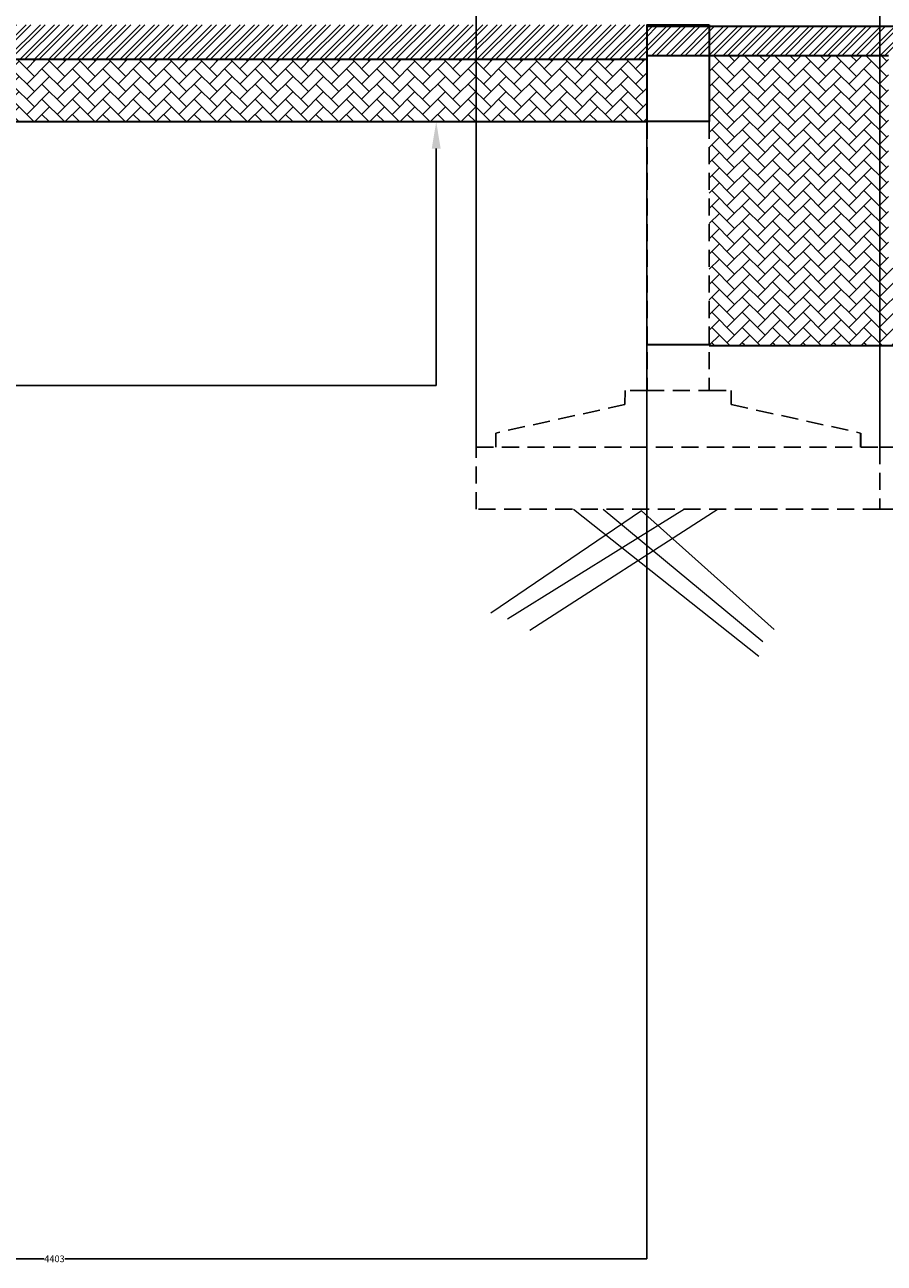
# Model space of a CAD drawing. Units: millimetres. Extents: x 1944 to 29915, y -10550 to 5909.
# Tile 19 of 24: x 22846 to 26040, y -10550 to -5946. Entities that reach past the tile are written whole.
import ezdxf
from ezdxf import colors
from ezdxf.entities.mleader import LeaderData, LeaderLine
from ezdxf.math import Vec2, Vec3

# ---------------------------------------------------------------- set-up
doc = ezdxf.new("R2010")
doc.units = ezdxf.units.MM
doc.header["$MEASUREMENT"] = 0
doc.linetypes.add('HIDDEN', pattern=[9.525, 6.35, -3.175])
for name, color, linetype, lineweight in [('A-ANNO-DIMS', 2, 'Continuous', 18), ('A-ANNO-TEXT', 7, 'Continuous', 25), ('A-FLOR-PATT', 252, 'Continuous', 13), ('A-SECT', 7, 'Continuous', 35), ('C-TOPO', 94, 'Continuous', 18), ('S-FNDN-HIDN', 1, 'HIDDEN', 25)]:
    doc.layers.add(name, color=color, linetype=linetype, lineweight=lineweight)
doc.styles.get("Standard").update_dxf_attribs({"font": 'arial.ttf'})
doc.dimstyles.get("Standard").update_dxf_attribs({"dimtxt": 25, "dimasz": 0.18, "dimexe": 0.18, "dimexo": 0.0625, "dimgap": 0.09, "dimtad": 0, "dimtih": 1, "dimtoh": 1, "dimdec": 0, "dimzin": 0, "dimdsep": 46, "dimtxsty": 'Standard', "dimcen": 0.09, "dimadec": 0, "dimazin": 0, "dimtfac": 1, "dimtdec": 0, "dimtofl": 0, "dimtmove": 0, "dimatfit": 3, "dimfxl": 1, "dimtolj": 1, "dimtzin": 0, "dimarcsym": 0})

# ---------------------------------------------------------------- blocks, each defined once
blk = doc.blocks.new('EARTH-COMPACT-SYMB')
for q in [(0, 60.9), (1053, 0)]:
    blk.add_line((559.8, 441.1), q)
blk = doc.blocks.new('*D89')
at = {"layer": 'A-ANNO-DIMS', "color": 0, "lineweight": -2, "transparency": 16777216}
for p, q in [((20755.4, -6305.8), (20755.4, -10533.3)), ((25158, -6305.8), (25158, -10533.3)), ((20755.6, -10533.1), (22918.8, -10533.1)), ((25157.8, -10533.1), (22994.7, -10533.1))]:
    blk.add_line(p, q, dxfattribs=at)
at = {"layer": 'A-ANNO-DIMS', "color": 0, "transparency": 16777216}
for points in [[(20755.6, -10533.1), (20755.6, -10533.1), (20755.4, -10533.1)], [(25157.8, -10533.1), (25157.8, -10533.1), (25158, -10533.1)]]:
    blk.add_solid(points, dxfattribs=at)
at = {"layer": 'Defpoints', "color": 0, "transparency": 16777216}
for p in [(20755.4, -6305.8), (25158, -6305.8), (25158, -10533.1)]:
    blk.add_point(p, dxfattribs=at)
at = {"layer": 'A-ANNO-DIMS', "color": 0, "transparency": 16777216, "insert": (22956.7, -10533.1), "char_height": 25, "attachment_point": 5}
blk.add_mtext('\\A1;4403', dxfattribs=at)
blk = doc.blocks.new('*D91')
at = {"layer": 'A-ANNO-DIMS', "color": 0, "lineweight": -2, "transparency": 16777216}
for p, q in [((24524.3, -7516.2), (24524.3, -395.6)), ((24524.5, -395.8), (25238.1, -395.8)), ((26024.1, -395.8), (25310.5, -395.8)), ((26024.3, -7516.2), (26024.3, -395.6))]:
    blk.add_line(p, q, dxfattribs=at)
at = {"layer": 'A-ANNO-DIMS', "color": 0, "transparency": 16777216}
for points in [[(24524.5, -395.7), (24524.5, -395.8), (24524.3, -395.8)], [(26024.1, -395.7), (26024.1, -395.8), (26024.3, -395.8)]]:
    blk.add_solid(points, dxfattribs=at)
at = {"layer": 'Defpoints', "color": 0, "transparency": 16777216}
for p in [(26024.3, -395.8), (24524.3, -7516.2), (26024.3, -7516.2)]:
    blk.add_point(p, dxfattribs=at)
at = {"layer": 'A-ANNO-DIMS', "color": 0, "transparency": 16777216, "insert": (25274.3, -395.8), "char_height": 25, "attachment_point": 5}
blk.add_mtext('\\A1;1500', dxfattribs=at)
blk = doc.blocks.new('*D92')
at = {"layer": 'A-ANNO-DIMS', "color": 0, "lineweight": -2, "transparency": 16777216}
for p, q in [((26024.4, -7516.2), (29886.4, -7516.2)), ((29886.2, -7516.4), (29886.2, -7618.4)), ((29886.2, -7746), (29886.2, -7644.1)), ((26024.4, -7746.2), (29886.4, -7746.2))]:
    blk.add_line(p, q, dxfattribs=at)
at = {"layer": 'A-ANNO-DIMS', "color": 0, "transparency": 16777216}
for points in [[(29886.2, -7516.4), (29886.3, -7516.4), (29886.2, -7516.2)], [(29886.2, -7746), (29886.3, -7746), (29886.2, -7746.2)]]:
    blk.add_solid(points, dxfattribs=at)
at = {"layer": 'Defpoints', "color": 0, "transparency": 16777216}
for p in [(26024.3, -7516.2), (26024.3, -7746.2), (29886.2, -7746.2)]:
    blk.add_point(p, dxfattribs=at)
at = {"layer": 'A-ANNO-DIMS', "color": 0, "transparency": 16777216, "insert": (29886.2, -7631.2), "char_height": 25, "attachment_point": 5}
blk.add_mtext('\\A1;230', dxfattribs=at)

msp = doc.modelspace()

# ---------------------------------------------------------------- hatches: boundary and pattern name
at = {"layer": 'A-FLOR-PATT'}
h = msp.add_hatch(dxfattribs=at)
h.set_pattern_fill('ANSI32', color=256, scale=100)
h.paths.add_polyline_path([(25159.297, -5945.752), (20985.45, -5945.752), (20985.45, -6073.852), (25159.297, -6073.852)])
h = msp.add_hatch(dxfattribs=at)
h.set_pattern_fill('ANSI32', color=256, scale=100)
h.paths.add_polyline_path([(25158.02, -5950.967), (26236.262, -5950.967), (26332.914, -6053.056), (26056.262, -6061.05), (25158.02, -6061.05)])
h = msp.add_hatch(dxfattribs=at)
h.set_pattern_fill('AR-HBONE', color=256, scale=10)
h.paths.add_polyline_path([(25159.297, -6073.852), (20985.45, -6073.852), (20985.45, -6305.752), (25159.297, -6305.752)])
h = msp.add_hatch(dxfattribs=at)
h.set_pattern_fill('AR-HBONE', color=256, scale=10)
h.paths.add_polyline_path([(25389.297, -6305.752), (25389.297, -6061.05), (26056.262, -6061.05), (26056.262, -6850.967), (26236.262, -6850.967), (27005.891, -6850.967), (27005.891, -6990.545), (26995.108, -6990.545), (26995.108, -7135.877), (25389.297, -7135.877)])

# ---------------------------------------------------------------- linework, layer by layer
at = {"layer": 'A-SECT'}
for p, q in [((25158.02, -5950.967), (26236.262, -5950.967)), ((20985.45, -6073.852), (25159.297, -6073.852)), ((26056.262, -6061.05), (25158.02, -6061.05)), ((20985.45, -6305.752), (25159.297, -6305.752)), ((25389.297, -7135.877), (25158.02, -7135.877)), ((27005.891, -7139.615), (25389.297, -7139.615)), ((25951.921, -7463.338), (25951.921, -7516.218))]:
    msp.add_line(p, q, dxfattribs=at)
msp.add_lwpolyline([(25389.297, -5945.752), (25389.297, -6305.752), (25159.297, -6305.752), (25159.297, -5945.752), (25389.297, -5945.752)], dxfattribs=at)
at = {"layer": 'C-TOPO'}
for p, q in [((25298.094, -7746.218), (24639.796, -8155.847)), ((25423.049, -7746.218), (24723.607, -8196.963)), ((24885.134, -7746.218), (25573.909, -8292.9)), ((24996.374, -7746.218), (25589.148, -8238.079))]:
    msp.add_line(p, q, dxfattribs=at)
at = {"layer": 'S-FNDN-HIDN', "ltscale": 10}
for p, q in [((25158.02, -6305.752), (25158.02, -7305.752)), ((25159.297, -6305.752), (25159.297, -7305.752)), ((25389.297, -6305.752), (25389.297, -7305.752)), ((25077.268, -7304.748), (25076.626, -7357.264)), ((25159.297, -7305.752), (25077.268, -7304.748)), ((25158.02, -7305.752), (25240.049, -7304.748)), ((25159.297, -7305.752), (25389.297, -7305.752)), ((25389.297, -7305.752), (25471.326, -7304.748)), ((25471.326, -7304.748), (25471.968, -7357.264)), ((25076.626, -7357.264), (24596.673, -7463.338)), ((25471.968, -7357.264), (25951.921, -7463.338)), ((24596.673, -7463.338), (24596.673, -7516.218))]:
    msp.add_line(p, q, dxfattribs=at)
msp.add_lwpolyline([(24524.297, -7516.218), (26024.297, -7516.218), (26024.297, -7746.218), (24524.297, -7746.218)], close=True, dxfattribs=at)

# ---------------------------------------------------------------- block references
at = {"layer": 'C-TOPO'}
msp.add_blockref('EARTH-COMPACT-SYMB', (24578.843, -8193.917), dxfattribs=at)

# ---------------------------------------------------------------- dimensions: what is measured, and where the dimension line sits
at = {"layer": 'A-ANNO-DIMS'}
for base, p1, p2, picture, middle in [((26024.297, -395.752), (24524.297, -7516.218), (26024.297, -7516.218), '*D91', (25274.297, -395.752)), ((25158.02, -10533.115), (20755.45, -6305.752), (25158.02, -6305.752), '*D89', (22956.735, -10533.115))]:
    dim = msp.add_linear_dim(base=base, p1=p1, p2=p2, dimstyle='Standard', override={"dimdec": 0, "dimlfac": 1, "dimrnd": 0, "dimzin": 0, "dimdsep": 46, "dimlunit": 2}, dxfattribs=at)
    dim.commit()
    dim.dimension.update_dxf_attribs({"geometry": picture, "text_midpoint": middle})
dim = msp.add_linear_dim(base=(29886.248, -7746.218), p1=(26024.297, -7516.218), p2=(26024.297, -7746.218), angle=90, dimstyle='Standard', override={"dimdec": 0, "dimlfac": 1, "dimrnd": 0, "dimzin": 0, "dimdsep": 46, "dimlunit": 2}, dxfattribs=at)
dim.commit()
dim.dimension.update_dxf_attribs({"geometry": '*D92', "text_midpoint": (29886.248, -7631.218)})

# ---------------------------------------------------------------- leaders
at = {"layer": 'A-ANNO-TEXT'}
ml = msp.add_multileader_mtext('Standard', dxfattribs=at)
ml.set_content('COMPACTED EARETH ', color=256)
ml.set_leader_properties()
ml.build(insert=Vec2(0, 0))
ml.multileader.update_dxf_attribs({"dogleg_length": 568.936, "arrow_head_size": 100})
ctx = ml.context
ctx.base_point, ctx.char_height, ctx.arrow_head_size, ctx.landing_gap_size, ctx.plane_origin = Vec3(21177.361, -7286.495), 100, 100, 0.09, Vec3(23226.285, -7286.495)
ctx.text_align_type = 2
notes = []
notes.append((ctx, [(0, (1, 1, 0), (23226.285, -7286.495), (-1, 0), 568.936, [(0, [(24375.34, -6305.752), (24375.34, -7286.495)], 0, [])])]))
ctx.mtext.insert, ctx.mtext.alignment, ctx.mtext.flow_direction = Vec3(22657.26, -7235.642), 3, 5
for ctx, leaders in notes:
    for number, flags, end, landing, length, lines in leaders:
        leader = LeaderData()
        leader.index, (leader.has_last_leader_line, leader.has_dogleg_vector, leader.attachment_direction) = number, flags
        leader.last_leader_point, leader.dogleg_vector, leader.dogleg_length = Vec3(end), Vec3(landing), length
        for number, points, colour, breaks in lines:
            line = LeaderLine()
            line.index, line.vertices, line.color, line.breaks = number, Vec3.list(points), colors.encode_raw_color(colour), breaks
            leader.lines.append(line)
        ctx.leaders.append(leader)

doc.saveas('drawing.dxf')
